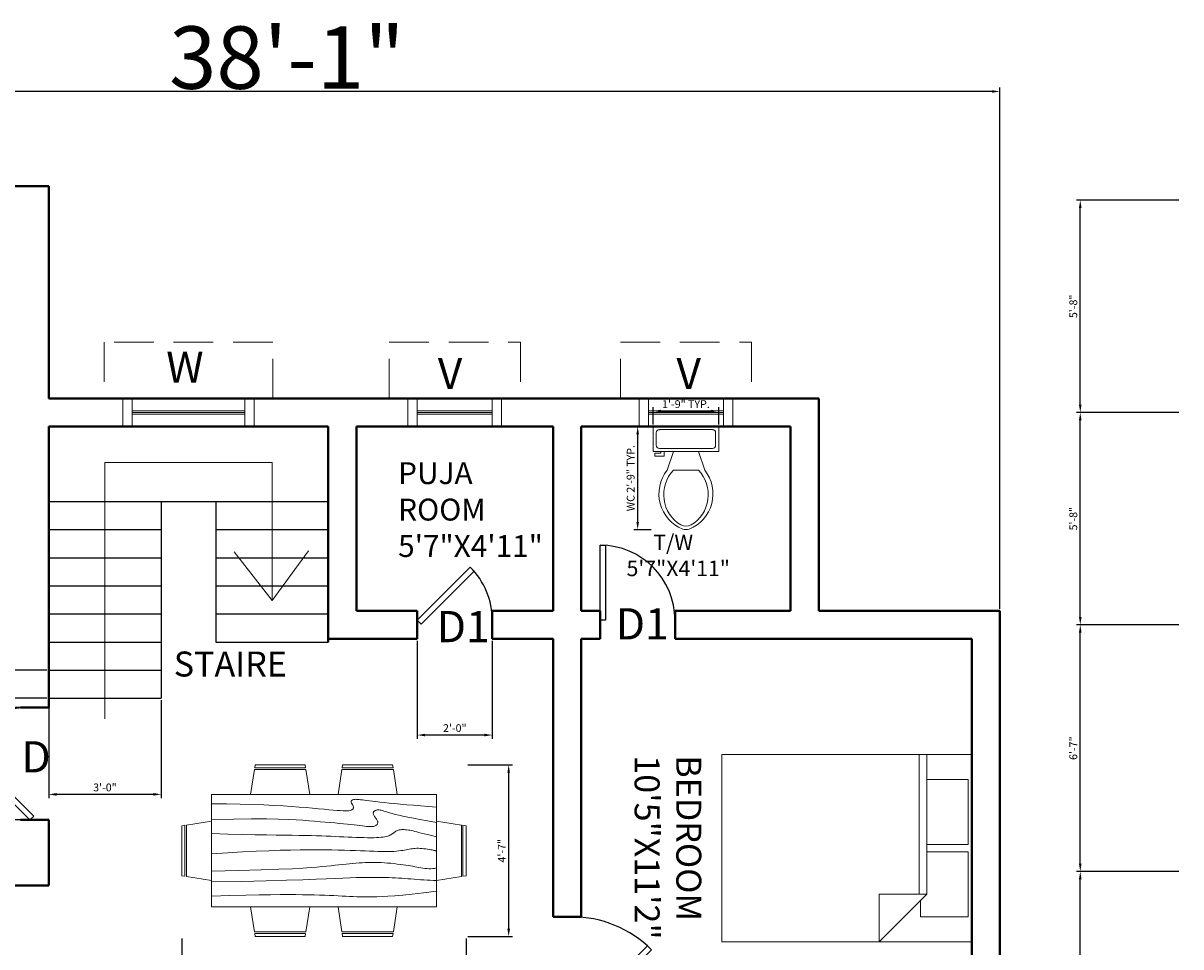
# Model space of a CAD drawing. Units: inches. Extents: x 4878 to 9282, y 5367 to 6617.
# Tile 6 of 14: x 5133 to 5503, y 6075 to 6371. Entities that reach past the tile are written whole.
import ezdxf

# ---------------------------------------------------------------- set-up
doc = ezdxf.new("R2010")
doc.units = ezdxf.units.IN
doc.linetypes.add('DASHED', pattern=[19.05, 12.7, -6.35])
for name, color, linetype, lineweight in [('A-ANNO-DIMS', 2, 'Continuous', 18), ('A-ANNO-SYMB', 2, 'Continuous', 18), ('A-ANNO-TEXT', 7, 'Continuous', 18), ('A-AREA-IDEN', 4, 'Continuous', 18), ('A-DOOR', 3, 'Continuous', 25), ('A-FLOR-FIXT', 9, 'Continuous', 20), ('A-FLOR-STRS', 7, 'Continuous', 25), ('A-FURN', 8, 'Continuous', 18), ('A-GLAZ', 30, 'Continuous', 20), ('A-ROOF-OVHD', 8, 'DASHED', 13), ('A-WALL', 7, 'Continuous', 40)]:
    doc.layers.add(name, color=color, linetype=linetype, lineweight=lineweight)
doc.styles.get("Standard").update_dxf_attribs({"font": 'arial.ttf'})
doc.dimstyles.new('ISO-25', dxfattribs={"dimtxt": 2.5, "dimasz": 2.5, "dimexe": 1.25, "dimexo": 0.625, "dimtad": 1, "dimdec": 0, "dimlunit": 3, "dimtxsty": 'Standard', "dimcen": 2.5, "dimadec": 0, "dimazin": 0, "dimtfac": 1, "dimtdec": 0, "dimtmove": 0, "dimatfit": 3, "dimfxl": 1, "dimarcsym": 0})

# ---------------------------------------------------------------- blocks, each defined once
blk = doc.blocks.new('Dining Set - 36 x 72 in.')
for p, q in [((-22.2343, 26.00059), (-23.4847, 17.99762)), ((-22.2304, 26), (-5.7608, 26)), ((-22, 27.5), (-22.1562, 26.50042)), ((-5.8416, 26.5), (-22.1534, 26.5)), ((-22, 27.5), (-6, 27.5)), ((-5.8437, 26.49966), (-6, 27.5)), ((-4.5152, 17.99762), (-5.7655, 25.99926)), ((5.7657, 26.00059), (4.5153, 17.99762)), ((5.7696, 26), (22.2392, 26)), ((6, 27.5), (5.8438, 26.50042)), ((22.1584, 26.5), (5.8466, 26.5)), ((6, 27.5), (22, 27.5)), ((22.1563, 26.49966), (22, 27.5)), ((23.4848, 17.99762), (22.2345, 25.99926)), ((36, 18), (-36, 18)), ((-36, 18), (-36, -18)), ((36, -18), (36, 18)), ((-45.5, 8), (-44.5004, 8.15617)), ((-45.5, 8), (-45.5, -8)), ((-44.5, -8.15843), (-44.5, 8.15338)), ((-44.0006, 8.23428), (-35.9976, 9.48474)), ((-44, 8.23041), (-44, -8.23915)), ((44.0006, 8.23428), (35.9976, 9.48474)), ((44, 8.23041), (44, -8.23915)), ((44.5, -8.15843), (44.5, 8.15338)), ((45.5, 8), (44.5005, 8.15617)), ((45.5, 8), (45.5, -8)), ((-44.4997, -8.15631), (-45.5, -8)), ((-35.9976, -9.48476), (-43.9993, -8.2345)), ((35.9976, -9.48476), (43.9993, -8.2345)), ((44.4997, -8.15631), (45.5, -8)), ((-36, -18), (36, -18)), ((-22.2343, -26.0006), (-23.4847, -17.99762)), ((-4.5152, -17.99762), (-5.7655, -25.99928)), ((5.7657, -26.0006), (4.5153, -17.99762)), ((23.4848, -17.99762), (22.2345, -25.99928)), ((-22.2304, -26), (-5.7608, -26)), ((-22, -27.5), (-22.1562, -26.50044)), ((-5.8416, -26.5), (-22.1534, -26.5)), ((-22, -27.5), (-6, -27.5)), ((-5.8437, -26.49967), (-6, -27.5)), ((5.7696, -26), (22.2392, -26)), ((6, -27.5), (5.8438, -26.50044)), ((22.1584, -26.5), (5.8466, -26.5)), ((6, -27.5), (22, -27.5)), ((22.1563, -26.49967), (22, -27.5))]:
    blk.add_line(p, q)
for points in [[(-36, 15), (-31.1772, 14.97754), (-26.8079, 14.91406), (-22.8538, 14.81543), (-19.276, 14.6875), (-16.0362, 14.53613), (-13.0957, 14.36718), (-10.4159, 14.18652), (-7.9583, 14), (-5.6904, 13.81315), (-3.6035, 13.63021), (-1.6954, 13.45508), (0.0365, 13.29166), (1.5945, 13.14388), (2.9811, 13.01562), (4.1988, 12.9108), (5.25, 12.83333), (6.1393, 12.78613), (6.8802, 12.76823), (7.4883, 12.77767), (7.9792, 12.8125), (8.3685, 12.87077), (8.6719, 12.95052), (8.9049, 13.0498), (9.0833, 13.16666), (9.2205, 13.29899), (9.3216, 13.44401), (9.3895, 13.59879), (9.4271, 13.76041), (9.4373, 13.92594), (9.4232, 14.09245), (9.3875, 14.257), (9.3333, 14.41666), (9.2638, 14.56917), (9.1836, 14.71484), (9.0975, 14.85465), (9.0104, 14.98958), (8.9272, 15.1206), (8.8529, 15.2487), (8.7922, 15.37483), (8.75, 15.5), (8.7305, 15.62467), (8.7344, 15.74739), (8.7617, 15.86621), (8.8125, 15.97916), (8.8867, 16.08431), (8.9844, 16.17968), (9.1055, 16.26334), (9.25, 16.33333), (9.4189, 16.38802), (9.6172, 16.42708), (9.8506, 16.45052), (10.125, 16.45833), (10.4463, 16.45052), (10.8203, 16.42708), (11.2529, 16.38802), (11.75, 16.33333), (12.3184, 16.26318), (12.9694, 16.17838), (13.7151, 16.07991), (14.5677, 15.96875), (15.5395, 15.84586), (16.6426, 15.71224), (17.8893, 15.56884), (19.2917, 15.41666), (20.859, 15.25667), (22.5879, 15.08984), (24.4721, 14.91715), (26.5052, 14.73958), (28.6809, 14.5581), (30.9929, 14.3737), (33.4347, 14.18733), (36, 14)], [(-36, 10), (-28.9766, 10.14274), (-23.1725, 10.20442), (-18.4241, 10.19775), (-14.5677, 10.13541), (-11.4399, 10.03011), (-8.877, 9.89453), (-6.7154, 9.74137), (-4.7917, 9.58333), (-2.9698, 9.43082), (-1.2246, 9.28515), (0.4415, 9.14534), (2.026, 9.01041), (3.5266, 8.87939), (4.9408, 8.7513), (6.266, 8.62516), (7.5, 8.5), (8.6411, 8.37549), (9.6914, 8.2539), (10.6538, 8.13818), (11.5312, 8.03125), (12.3267, 7.93603), (13.043, 7.85547), (13.6831, 7.79248), (14.25, 7.75), (14.7471, 7.7303), (15.1797, 7.73307), (15.5537, 7.75732), (15.875, 7.80208), (16.1494, 7.86637), (16.3828, 7.94922), (16.5811, 8.04964), (16.75, 8.16666), (16.8944, 8.29915), (17.0143, 8.44531), (17.1089, 8.60319), (17.1771, 8.77083), (17.218, 8.94629), (17.2305, 9.1276), (17.2137, 9.31282), (17.1667, 9.5), (17.0895, 9.6875), (16.987, 9.875), (16.8649, 10.0625), (16.7292, 10.25), (16.5856, 10.4375), (16.4401, 10.625), (16.2985, 10.8125), (16.1667, 11), (16.05, 11.18733), (15.9518, 11.3737), (15.8752, 11.5581), (15.8229, 11.73958), (15.798, 11.91715), (15.8034, 12.08984), (15.842, 12.25667), (15.9167, 12.41666), (16.0295, 12.56836), (16.1784, 12.70833), (16.3605, 12.83268), (16.5729, 12.9375), (16.8127, 13.01888), (17.0768, 13.07291), (17.3625, 13.0957), (17.6667, 13.08333), (17.9894, 13.03312), (18.3418, 12.94726), (18.7382, 12.82918), (19.1927, 12.68229), (19.7195, 12.51001), (20.3327, 12.31575), (21.0465, 12.10294), (21.875, 11.875), (22.8357, 11.63354), (23.959, 11.37304), (25.2786, 11.08618), (26.8282, 10.76562), (28.6414, 10.40405), (30.752, 9.99414), (33.1936, 9.52856), (36, 9)], [(-36, 5.5), (-30.7157, 5.3348), (-26.069, 5.20963), (-21.9946, 5.11767), (-18.4271, 5.05208), (-15.3009, 5.00602), (-12.5508, 4.97265), (-10.1112, 4.94515), (-7.9167, 4.91666), (-5.909, 4.88167), (-4.0586, 4.83984), (-2.3429, 4.79215), (-0.7396, 4.73958), (0.7739, 4.6831), (2.22, 4.6237), (3.6213, 4.56233), (5, 4.5), (6.373, 4.43782), (7.7344, 4.3776), (9.0723, 4.32129), (10.375, 4.27083), (11.6309, 4.22819), (12.8281, 4.19531), (13.9551, 4.17415), (15, 4.16666), (15.954, 4.17448), (16.819, 4.19791), (17.6001, 4.23698), (18.3021, 4.29166), (18.9299, 4.36198), (19.4883, 4.44791), (19.9823, 4.54948), (20.4167, 4.66666), (20.7969, 4.79899), (21.1302, 4.94401), (21.4245, 5.09879), (21.6875, 5.26041), (21.9271, 5.42594), (22.1511, 5.59245), (22.3672, 5.757), (22.5834, 5.91666), (22.8065, 6.06868), (23.0404, 6.21093), (23.2879, 6.34147), (23.5521, 6.45833), (23.8358, 6.55957), (24.142, 6.64323), (24.4735, 6.70735), (24.8334, 6.75), (25.2235, 6.76969), (25.642, 6.76692), (26.0858, 6.74267), (26.5521, 6.69791), (27.0379, 6.63362), (27.5404, 6.55078), (28.0565, 6.45036), (28.5834, 6.33333), (29.1242, 6.19987), (29.7071, 6.04687), (30.3661, 5.87044), (31.1354, 5.66666), (32.0493, 5.43164), (33.142, 5.16146), (34.4475, 4.85221), (36, 4.5)], [(-36, -1), (-30.7915, -0.6591), (-26.0195, -0.38216), (-21.6519, -0.16284), (-17.6563, 0.00521), (-14.0005, 0.12833), (-10.6523, 0.21289), (-7.5796, 0.26522), (-4.75, 0.29166), (-2.134, 0.29793), (0.2878, 0.28711), (2.5317, 0.26163), (4.6146, 0.22396), (6.5529, 0.17651), (8.3633, 0.12174), (10.0623, 0.06209), (11.6667, 0), (13.1899, -0.06201), (14.6341, -0.1211), (15.9982, -0.17432), (17.2813, -0.21875), (18.4823, -0.25147), (19.6003, -0.26953), (20.6343, -0.27002), (21.5834, -0.25), (22.4481, -0.20768), (23.2357, -0.14584), (23.9549, -0.06836), (24.6146, 0.02083), (25.2235, 0.11784), (25.7904, 0.21875), (26.3241, 0.31966), (26.8334, 0.41666), (27.3265, 0.50618), (27.8099, 0.58593), (28.2894, 0.65397), (28.7709, 0.70833), (29.2601, 0.74707), (29.763, 0.76823), (30.2855, 0.76985), (30.8334, 0.75), (31.4088, 0.70784), (31.9994, 0.64713), (32.589, 0.57275), (33.1615, 0.48958), (33.7008, 0.4025), (34.1908, 0.3164), (34.6153, 0.23616), (34.9584, 0.16666), (35.2099, 0.11165), (35.3848, 0.07031), (35.504, 0.04069), (35.5886, 0.02083), (35.6594, 0.00879), (35.7377, 0.0026), (35.8442, 0.00032), (36, 0)], [(-36, -6.5), (-27.1843, -6.31267), (-20.084, -6.1263), (-14.469, -5.9419), (-10.1094, -5.76042), (-6.7752, -5.58285), (-4.2363, -5.41016), (-2.2629, -5.24333), (-0.625, -5.08334), (0.8708, -4.93099), (2.2715, -4.78646), (3.5872, -4.64974), (4.8281, -4.52084), (6.0046, -4.39974), (7.127, -4.28646), (8.2053, -4.18099), (9.25, -4.08334), (10.2705, -3.99382), (11.2734, -3.91407), (12.2647, -3.84603), (13.25, -3.79167), (14.2354, -3.75293), (15.2266, -3.73177), (16.2295, -3.73015), (17.25, -3.75), (18.2912, -3.79248), (19.3451, -3.85547), (20.4009, -3.93604), (21.4479, -4.03125), (22.4754, -4.13819), (23.4727, -4.25391), (24.4289, -4.37549), (25.3334, -4.5), (26.1785, -4.62492), (26.9694, -4.74935), (27.7145, -4.87281), (28.4219, -4.99479), (29.1, -5.11483), (29.7572, -5.23242), (30.4016, -5.34709), (31.0417, -5.45834), (31.6837, -5.56437), (32.3262, -5.65821), (32.9658, -5.73153), (33.599, -5.77604), (34.2224, -5.78345), (34.8327, -5.74545), (35.4264, -5.65373), (36, -5.5)], [(-36, -10), (-26.4022, -9.81299), (-18.4675, -9.62891), (-11.9839, -9.45069), (-6.7396, -9.28125), (-2.5226, -9.12354), (0.8789, -8.98047), (3.6769, -8.85498), (6.0833, -8.75), (8.2767, -8.66765), (10.3021, -8.60677), (12.1712, -8.56543), (13.8958, -8.54167), (15.4876, -8.53353), (16.9583, -8.53907), (18.3197, -8.55632), (19.5834, -8.58334), (20.7616, -8.61841), (21.8685, -8.66081), (22.9188, -8.71004), (23.9271, -8.76563), (24.9081, -8.82707), (25.8763, -8.89388), (26.8465, -8.96558), (27.8334, -9.04167), (28.8474, -9.12118), (29.8828, -9.20117), (30.93, -9.27824), (31.9792, -9.34896), (33.0205, -9.40991), (34.0443, -9.45768), (35.0407, -9.48885), (36, -9.5)], [(-36, -14.5), (-30.0881, -14.33513), (-25.0332, -14.21224), (-20.7312, -14.12647), (-17.0781, -14.07292), (-13.97, -14.04671), (-11.3027, -14.04297), (-8.9724, -14.05681), (-6.875, -14.08334), (-4.9224, -14.11833), (-3.0905, -14.16016), (-1.3709, -14.20785), (0.2448, -14.26042), (1.7647, -14.3169), (3.1973, -14.3763), (4.5507, -14.43767), (5.8333, -14.5), (7.0554, -14.5621), (8.235, -14.62175), (9.3922, -14.67652), (10.5469, -14.72396), (11.7192, -14.76164), (12.929, -14.78711), (14.1965, -14.79794), (15.5417, -14.79167), (16.9933, -14.76424), (18.6152, -14.70508), (20.4804, -14.60197), (22.6615, -14.44271), (25.2312, -14.21509), (28.2624, -13.9069), (31.8277, -13.50594), (36, -13)]]:
    blk.add_lwpolyline(points)
blk = doc.blocks.new('Bed - Queen')
for p, q in [((0, -80.00003), (0, 0)), ((0, 0), (59.99999, 0)), ((59.99999, 0), (59.99999, -80.00003)), ((7.99999, -1.2), (28.79998, -1.2)), ((7.99999, -14.4), (7.99999, -1.2)), ((28.79998, -1.2), (28.79998, -14.4)), ((31.19999, -1.2), (51.99999, -1.2)), ((31.19999, -14.4), (31.19999, -1.2)), ((51.99999, -1.2), (51.99999, -16.4)), ((0, -14.4), (44.8, -14.4)), ((59.99999, -29.6), (44.8, -14.4)), ((44.8, -14.4), (44.8, -29.6)), ((44.8, -16.8), (0, -16.8)), ((51.99999, -16.4), (46.79936, -16.4)), ((44.8, -29.6), (59.99999, -29.6)), ((59.99999, -80.00003), (0, -80.00003))]:
    blk.add_line(p, q)
blk = doc.blocks.new('Toilet - top')
for p, q in [((9.5, -6), (9.5, -2)), ((-10, -8.5), (-8, -8.5)), ((-10, -9.5), (-10, -8.5)), ((-7, -9.5), (-10, -9.5)), ((-8, -8.5), (-8, -8)), ((-7, -8), (-7, -9.5)), ((-4, -8), (-6, -14)), ((4, -8), (6, -14)), ((4, -14), (-4, -14))]:
    blk.add_line(p, q)
blk.add_lwpolyline([(10.5, -8), (10.5, 0), (-10.5, 0), (-10.5, -8)], close=True)
for points in [[(-9.5, -2), (-9.5, -6)], [(8.5, -1), (-8.5, -1)], [(-8.5, -7), (8.5, -7)]]:
    blk.add_lwpolyline(points)
for centre, radius, start, end in [((-8.62, -1.88), 0.884, 81.8699, 188.1301), ((8.62, -1.88), 0.884, 351.8699, 98.1301), ((-8.62, -6.12), 0.884, 171.8699, 278.1301), ((8.62, -6.12), 0.884, 261.8699, 8.1301), ((3.52, -21.58), 12.17, 141.4691, 247.9714), ((4.2, -21.82), 11.33, 136.3677, 238.9468), ((-3.52, -21.58), 12.17, 292.0284, 38.5307), ((-4.2, -21.82), 11.33, 301.053, 43.6321), ((0, -27.88), 4, 245.7318, 294.2682), ((0, -29), 4, 254.8605, 285.1395)]:
    blk.add_arc(centre, radius, start, end)
blk = doc.blocks.new('*U10')
for p, q in [((0, 0), (0, -6)), ((24, 0), (24, -6))]:
    blk.add_line(p, q)
blk.add_lwpolyline([(0, 0), (16.97, 16.97), (18.21, 15.73), (1.24, -1.24)], close=True)
blk.add_arc((0, 0), 24, 0, 45)
blk = doc.blocks.new('*U15')
for p, q in [((0, 0), (0, -6)), ((24, 0), (24, -6))]:
    blk.add_line(p, q)
blk.add_lwpolyline([(0, 0), (0, 24), (1.75, 24), (1.75, 0)], close=True)
blk.add_arc((0, 0), 24, 0, 90)
blk = doc.blocks.new('*U8')
for p, q in [((-36, 0), (-36, 6)), ((0, 0), (0, 6))]:
    blk.add_line(p, q)
blk.add_lwpolyline([(0, 0), (-25.46, -25.46), (-26.69, -24.22), (-1.24, 1.24)], close=True)
blk.add_arc((0, 0), 36, 180, 225)
blk = doc.blocks.new('*U13')
for p, q in [((0, 0), (0, -6)), ((-36, 0), (-36, -6))]:
    blk.add_line(p, q)
blk.add_lwpolyline([(0, 0), (-25.46, 25.46), (-26.69, 24.22), (-1.24, -1.24)], close=True)
blk.add_arc((0, 0), 36, 135, 180)
blk = doc.blocks.new('*D16')
at = {"layer": 'A-ANNO-DIMS', "color": 0, "lineweight": -2, "transparency": 16777216}
for p, q in [((4988.98, 6183.27), (4988.98, 6350.19)), ((5442.98, 6348.94), (4991.48, 6348.94)), ((5445.48, 6183.27), (5445.48, 6350.19))]:
    blk.add_line(p, q, dxfattribs=at)
at = {"layer": 'A-ANNO-DIMS', "color": 0, "transparency": 16777216}
for points in [[(4991.48, 6349.36), (4991.48, 6348.53), (4988.98, 6348.94)], [(5442.98, 6349.36), (5442.98, 6348.53), (5445.48, 6348.94)]]:
    blk.add_solid(points, dxfattribs=at)
at = {"layer": 'Defpoints', "color": 0, "transparency": 16777216}
for p in [(4988.98, 6348.94), (4988.98, 6182.64), (5445.48, 6182.64)]:
    blk.add_point(p, dxfattribs=at)
at = {"layer": 'A-ANNO-DIMS', "color": 0, "transparency": 16777216, "insert": (5217.23, 6359.79), "char_height": 2.5, "attachment_point": 5}
blk.add_mtext('{\\H8x;38\'-1"}', dxfattribs=at)
blk = doc.blocks.new('WINDOW-PLAN-36IN')
for p, q in [((0, 0), (0, 9)), ((3, 0), (3, 9)), ((39, 0), (39, 9)), ((42, 0), (42, 9)), ((3, 5), (39, 5)), ((3, 4.5), (39, 4.5)), ((3, 4), (39, 4))]:
    blk.add_line(p, q)
blk = doc.blocks.new('WINDOW-PLAN-24IN')
for p, q in [((9, 30), (0, 30)), ((9, 27), (0, 27)), ((4, 3), (4, 27)), ((4.5, 3), (4.5, 27)), ((5, 3), (5, 27)), ((9, 3), (0, 3)), ((9, 0), (0, 0))]:
    blk.add_line(p, q)
blk = doc.blocks.new('WINDOW-HOOD-54IN')
for p, q in [((0, 18), (0, 0)), ((54, 0), (54, 18)), ((0, 0), (54, 0))]:
    blk.add_line(p, q)
blk = doc.blocks.new('WINDOW-HOOD-42IN')
for p, q in [((18, 42), (0, 42)), ((0, 42), (0, 0)), ((0, 0), (18, 0))]:
    blk.add_line(p, q)
blk = doc.blocks.new('*D55')
at = {"layer": 'A-ANNO-DIMS', "color": 0, "lineweight": -2, "transparency": 16777216}
for p, q in [((5333.85, 6241.64), (5328.27, 6241.64)), ((5329.52, 6211.1), (5329.52, 6239.14)), ((5333.85, 6208.6), (5328.27, 6208.6))]:
    blk.add_line(p, q, dxfattribs=at)
at = {"layer": 'A-ANNO-DIMS', "color": 0, "transparency": 16777216}
for points in [[(5329.1, 6239.14), (5329.94, 6239.14), (5329.52, 6241.64)], [(5329.1, 6211.1), (5329.94, 6211.1), (5329.52, 6208.6)]]:
    blk.add_solid(points, dxfattribs=at)
at = {"layer": 'Defpoints', "color": 0, "transparency": 16777216}
for p in [(5329.52, 6241.64), (5334.48, 6241.64), (5334.48, 6208.6)]:
    blk.add_point(p, dxfattribs=at)
at = {"layer": 'A-ANNO-DIMS', "color": 0, "transparency": 16777216, "insert": (5327.6, 6225.12), "char_height": 2.5, "attachment_point": 5, "rotation": 90}
blk.add_mtext('WC 2\'-9" TYP.', dxfattribs=at)
blk = doc.blocks.new('*D56')
at = {"layer": 'A-ANNO-DIMS', "color": 0, "lineweight": -2, "transparency": 16777216}
for p, q in [((5334.48, 6242.27), (5334.48, 6247.85)), ((5336.98, 6246.6), (5352.98, 6246.6)), ((5355.48, 6242.27), (5355.48, 6247.85))]:
    blk.add_line(p, q, dxfattribs=at)
at = {"layer": 'A-ANNO-DIMS', "color": 0, "transparency": 16777216}
for points in [[(5336.98, 6247.02), (5336.98, 6246.19), (5334.48, 6246.6)], [(5352.98, 6247.02), (5352.98, 6246.19), (5355.48, 6246.6)]]:
    blk.add_solid(points, dxfattribs=at)
at = {"layer": 'Defpoints', "color": 0, "transparency": 16777216}
for p in [(5355.48, 6246.6), (5334.48, 6241.64), (5355.48, 6241.64)]:
    blk.add_point(p, dxfattribs=at)
at = {"layer": 'A-ANNO-DIMS', "color": 0, "transparency": 16777216, "insert": (5344.98, 6248.5), "char_height": 2.5, "attachment_point": 5}
blk.add_mtext('1\'-9" TYP.', dxfattribs=at)
blk = doc.blocks.new('*D61')
at = {"layer": 'A-ANNO-DIMS', "color": 0, "lineweight": -2, "transparency": 16777216}
for p, q in [((5183.58, 6077.68), (5183.58, 6063.4)), ((5274.58, 6077.68), (5274.58, 6063.4)), ((5186.08, 6064.65), (5272.08, 6064.65))]:
    blk.add_line(p, q, dxfattribs=at)
at = {"layer": 'A-ANNO-DIMS', "color": 0, "transparency": 16777216}
for points in [[(5186.08, 6065.07), (5186.08, 6064.23), (5183.58, 6064.65)], [(5272.08, 6065.07), (5272.08, 6064.23), (5274.58, 6064.65)]]:
    blk.add_solid(points, dxfattribs=at)
at = {"layer": 'Defpoints', "color": 0, "transparency": 16777216}
for p in [(5183.58, 6078.3), (5274.58, 6078.3), (5274.58, 6064.65)]:
    blk.add_point(p, dxfattribs=at)
at = {"layer": 'A-ANNO-DIMS', "color": 0, "transparency": 16777216, "insert": (5229.08, 6066.57), "char_height": 2.5, "attachment_point": 5}
blk.add_mtext('DINING SET 7\'-7"', dxfattribs=at)
blk = doc.blocks.new('*D62')
at = {"layer": 'A-ANNO-DIMS', "color": 0, "lineweight": -2, "transparency": 16777216}
for p, q in [((5275.2, 6133.3), (5289.48, 6133.3)), ((5288.23, 6080.8), (5288.23, 6130.8)), ((5275.2, 6078.3), (5289.48, 6078.3))]:
    blk.add_line(p, q, dxfattribs=at)
at = {"layer": 'A-ANNO-DIMS', "color": 0, "transparency": 16777216}
for points in [[(5287.81, 6130.8), (5288.64, 6130.8), (5288.23, 6133.3)], [(5287.81, 6080.8), (5288.64, 6080.8), (5288.23, 6078.3)]]:
    blk.add_solid(points, dxfattribs=at)
at = {"layer": 'Defpoints', "color": 0, "transparency": 16777216}
for p in [(5274.58, 6133.3), (5288.23, 6133.3), (5274.58, 6078.3)]:
    blk.add_point(p, dxfattribs=at)
at = {"layer": 'A-ANNO-DIMS', "color": 0, "transparency": 16777216, "insert": (5286.35, 6105.8), "char_height": 2.5, "attachment_point": 5, "rotation": 90}
blk.add_mtext('4\'-7"', dxfattribs=at)
blk = doc.blocks.new('*D74')
at = {"layer": 'A-ANNO-DIMS', "color": 0, "lineweight": -2, "transparency": 16777216}
for p, q in [((5502.78, 6099.14), (5469.95, 6099.14)), ((5471.2, 6037.64), (5471.2, 6096.64)), ((5502.78, 6035.14), (5469.95, 6035.14))]:
    blk.add_line(p, q, dxfattribs=at)
at = {"layer": 'A-ANNO-DIMS', "color": 0, "transparency": 16777216}
for points in [[(5470.79, 6096.64), (5471.62, 6096.64), (5471.2, 6099.14)], [(5470.79, 6037.64), (5471.62, 6037.64), (5471.2, 6035.14)]]:
    blk.add_solid(points, dxfattribs=at)
at = {"layer": 'Defpoints', "color": 0, "transparency": 16777216}
for p in [(5471.2, 6099.14), (5503.4, 6099.14), (5503.4, 6035.14)]:
    blk.add_point(p, dxfattribs=at)
at = {"layer": 'A-ANNO-DIMS', "color": 0, "transparency": 16777216, "insert": (5469.31, 6067.14), "char_height": 2.5, "attachment_point": 5, "rotation": 90}
blk.add_mtext('5\'-4"', dxfattribs=at)
blk = doc.blocks.new('*D75')
at = {"layer": 'A-ANNO-DIMS', "color": 0, "lineweight": -2, "transparency": 16777216}
for p, q in [((5502.78, 6178.14), (5469.95, 6178.14)), ((5471.2, 6101.64), (5471.2, 6175.64)), ((5502.78, 6099.14), (5469.95, 6099.14))]:
    blk.add_line(p, q, dxfattribs=at)
at = {"layer": 'A-ANNO-DIMS', "color": 0, "transparency": 16777216}
for points in [[(5470.79, 6175.64), (5471.62, 6175.64), (5471.2, 6178.14)], [(5470.79, 6101.64), (5471.62, 6101.64), (5471.2, 6099.14)]]:
    blk.add_solid(points, dxfattribs=at)
at = {"layer": 'Defpoints', "color": 0, "transparency": 16777216}
for p in [(5471.2, 6178.14), (5503.4, 6178.14), (5503.4, 6099.14)]:
    blk.add_point(p, dxfattribs=at)
at = {"layer": 'A-ANNO-DIMS', "color": 0, "transparency": 16777216, "insert": (5469.3, 6138.64), "char_height": 2.5, "attachment_point": 5, "rotation": 90}
blk.add_mtext('6\'-7"', dxfattribs=at)
blk = doc.blocks.new('*D76')
at = {"layer": 'A-ANNO-DIMS', "color": 0, "lineweight": -2, "transparency": 16777216}
for p, q in [((5502.78, 6246.14), (5469.95, 6246.14)), ((5471.2, 6180.64), (5471.2, 6243.64)), ((5502.78, 6178.14), (5469.95, 6178.14))]:
    blk.add_line(p, q, dxfattribs=at)
at = {"layer": 'A-ANNO-DIMS', "color": 0, "transparency": 16777216}
for points in [[(5470.79, 6243.64), (5471.62, 6243.64), (5471.2, 6246.14)], [(5470.79, 6180.64), (5471.62, 6180.64), (5471.2, 6178.14)]]:
    blk.add_solid(points, dxfattribs=at)
at = {"layer": 'Defpoints', "color": 0, "transparency": 16777216}
for p in [(5471.2, 6246.14), (5503.4, 6246.14), (5503.4, 6178.14)]:
    blk.add_point(p, dxfattribs=at)
at = {"layer": 'A-ANNO-DIMS', "color": 0, "transparency": 16777216, "insert": (5469.3, 6212.14), "char_height": 2.5, "attachment_point": 5, "rotation": 90}
blk.add_mtext('5\'-8"', dxfattribs=at)
blk = doc.blocks.new('*D77')
at = {"layer": 'A-ANNO-DIMS', "color": 0, "lineweight": -2, "transparency": 16777216}
for p, q in [((5502.78, 6314.14), (5469.95, 6314.14)), ((5471.2, 6248.64), (5471.2, 6311.64)), ((5502.78, 6246.14), (5469.95, 6246.14))]:
    blk.add_line(p, q, dxfattribs=at)
at = {"layer": 'A-ANNO-DIMS', "color": 0, "transparency": 16777216}
for points in [[(5470.79, 6311.64), (5471.62, 6311.64), (5471.2, 6314.14)], [(5470.79, 6248.64), (5471.62, 6248.64), (5471.2, 6246.14)]]:
    blk.add_solid(points, dxfattribs=at)
at = {"layer": 'Defpoints', "color": 0, "transparency": 16777216}
for p in [(5471.2, 6314.14), (5503.4, 6314.14), (5503.4, 6246.14)]:
    blk.add_point(p, dxfattribs=at)
at = {"layer": 'A-ANNO-DIMS', "color": 0, "transparency": 16777216, "insert": (5469.3, 6280.14), "char_height": 2.5, "attachment_point": 5, "rotation": 90}
blk.add_mtext('5\'-8"', dxfattribs=at)
blk = doc.blocks.new('*D105')
at = {"layer": 'A-ANNO-DIMS', "color": 0, "lineweight": -2, "transparency": 16777216}
for p, q in [((5140.35, 6151.64), (5108.93, 6151.64)), ((5110.18, 6118.14), (5110.18, 6149.14)), ((5140.35, 6115.64), (5108.93, 6115.64))]:
    blk.add_line(p, q, dxfattribs=at)
at = {"layer": 'A-ANNO-DIMS', "color": 0, "transparency": 16777216}
for points in [[(5109.76, 6149.14), (5110.59, 6149.14), (5110.18, 6151.64)], [(5109.76, 6118.14), (5110.59, 6118.14), (5110.18, 6115.64)]]:
    blk.add_solid(points, dxfattribs=at)
at = {"layer": 'Defpoints', "color": 0, "transparency": 16777216}
for p in [(5110.18, 6151.64), (5140.98, 6151.64), (5140.98, 6115.64)]:
    blk.add_point(p, dxfattribs=at)
at = {"layer": 'A-ANNO-DIMS', "color": 0, "transparency": 16777216, "insert": (5108.27, 6133.64), "char_height": 2.5, "attachment_point": 5, "rotation": 90}
blk.add_mtext('3\'-0"', dxfattribs=at)
blk = doc.blocks.new('*D106')
at = {"layer": 'A-ANNO-DIMS', "color": 0, "lineweight": -2, "transparency": 16777216}
for p, q in [((5258.98, 6173.02), (5258.98, 6141.59)), ((5282.98, 6173.02), (5282.98, 6141.59)), ((5280.48, 6142.84), (5261.48, 6142.84))]:
    blk.add_line(p, q, dxfattribs=at)
at = {"layer": 'A-ANNO-DIMS', "color": 0, "transparency": 16777216}
for points in [[(5261.48, 6143.26), (5261.48, 6142.43), (5258.98, 6142.84)], [(5280.48, 6143.26), (5280.48, 6142.43), (5282.98, 6142.84)]]:
    blk.add_solid(points, dxfattribs=at)
at = {"layer": 'Defpoints', "color": 0, "transparency": 16777216}
for p in [(5258.98, 6173.64), (5282.98, 6173.64), (5258.98, 6142.84)]:
    blk.add_point(p, dxfattribs=at)
at = {"layer": 'A-ANNO-DIMS', "color": 0, "transparency": 16777216, "insert": (5270.98, 6144.75), "char_height": 2.5, "attachment_point": 5}
blk.add_mtext('2\'-0"', dxfattribs=at)
blk = doc.blocks.new('*D113')
at = {"layer": 'A-ANNO-DIMS', "color": 0, "lineweight": -2, "transparency": 16777216}
for p, q in [((5140.98, 6154.02), (5140.98, 6122.59)), ((5176.98, 6154.02), (5176.98, 6122.59)), ((5174.48, 6123.84), (5143.48, 6123.84))]:
    blk.add_line(p, q, dxfattribs=at)
at = {"layer": 'A-ANNO-DIMS', "color": 0, "transparency": 16777216}
for points in [[(5143.48, 6124.26), (5143.48, 6123.43), (5140.98, 6123.84)], [(5174.48, 6124.26), (5174.48, 6123.43), (5176.98, 6123.84)]]:
    blk.add_solid(points, dxfattribs=at)
at = {"layer": 'Defpoints', "color": 0, "transparency": 16777216}
for p in [(5140.98, 6154.64), (5176.98, 6154.64), (5140.98, 6123.84)]:
    blk.add_point(p, dxfattribs=at)
at = {"layer": 'A-ANNO-DIMS', "color": 0, "transparency": 16777216, "insert": (5158.98, 6125.75), "char_height": 2.5, "attachment_point": 5}
blk.add_mtext('3\'-0"', dxfattribs=at)
blk = doc.blocks.new('*D114')
at = {"layer": 'A-ANNO-DIMS', "color": 0, "lineweight": -2, "transparency": 16777216}
for p, q in [((5140.35, 6163.64), (4938.93, 6163.64)), ((4940.18, 6161.14), (4940.18, 6157.14)), ((5140.35, 6154.64), (4938.93, 6154.64))]:
    blk.add_line(p, q, dxfattribs=at)
at = {"layer": 'A-ANNO-DIMS', "color": 0, "transparency": 16777216}
for points in [[(4939.76, 6161.14), (4940.59, 6161.14), (4940.18, 6163.64)], [(4939.76, 6157.14), (4940.59, 6157.14), (4940.18, 6154.64)]]:
    blk.add_solid(points, dxfattribs=at)
at = {"layer": 'Defpoints', "color": 0, "transparency": 16777216}
for p in [(5140.98, 6163.64), (4940.18, 6154.64), (5140.98, 6154.64)]:
    blk.add_point(p, dxfattribs=at)
at = {"layer": 'A-ANNO-DIMS', "color": 0, "transparency": 16777216, "insert": (4938.28, 6159.14), "char_height": 2.5, "attachment_point": 5, "rotation": 90}
blk.add_mtext('0\'-9"', dxfattribs=at)

msp = doc.modelspace()

# ---------------------------------------------------------------- linework, layer by layer
at = {"layer": 'A-ANNO-SYMB'}
for p, q in [((5158.98, 6148.02), (5158.98, 6230.17)), ((5158.98, 6230.17), (5212.48, 6230.17)), ((5212.48, 6230.17), (5212.48, 6185.94)), ((5212.48, 6185.94), (5200.37, 6201.49)), ((5212.48, 6185.94), (5224.12, 6201.83))]:
    msp.add_line(p, q, dxfattribs=at)
at = {"layer": 'A-FLOR-STRS'}
for p, q in [((5140.98, 6217.64), (5230.48, 6217.64)), ((5176.98, 6217.64), (5176.98, 6154.64)), ((5194.48, 6217.64), (5194.48, 6172.64)), ((5140.98, 6208.64), (5176.98, 6208.64)), ((5194.48, 6208.64), (5230.48, 6208.64)), ((5140.98, 6199.64), (5176.98, 6199.64)), ((5194.48, 6199.64), (5230.48, 6199.64)), ((5140.98, 6190.64), (5176.98, 6190.64)), ((5194.48, 6190.64), (5230.48, 6190.64)), ((5140.98, 6181.64), (5176.98, 6181.64)), ((5194.48, 6181.64), (5230.48, 6181.64)), ((5140.98, 6172.64), (5176.98, 6172.64)), ((5194.48, 6172.64), (5230.48, 6172.64)), ((5140.98, 6163.64), (5176.98, 6163.64)), ((5140.98, 6154.64), (5176.98, 6154.64))]:
    msp.add_line(p, q, dxfattribs=at)
at = {"layer": 'A-WALL'}
for p, q in [((5043.98, 6318.64), (5140.98, 6318.64)), ((5140.98, 6318.64), (5140.98, 6250.64)), ((5140.98, 6250.64), (5387.48, 6250.64)), ((5387.48, 6250.64), (5387.48, 6182.64)), ((5140.98, 6241.64), (5230.48, 6241.64)), ((5140.98, 6241.64), (5140.98, 6151.64)), ((5230.48, 6241.64), (5230.48, 6172.64)), ((5239.48, 6241.64), (5239.48, 6182.64)), ((5239.48, 6241.64), (5302.48, 6241.64)), ((5302.48, 6241.64), (5302.48, 6182.64)), ((5311.48, 6241.64), (5311.48, 6182.64)), ((5311.48, 6241.64), (5378.48, 6241.64)), ((5378.48, 6241.64), (5378.48, 6182.64)), ((5239.48, 6182.64), (5258.98, 6182.64)), ((5258.98, 6182.64), (5258.98, 6173.64)), ((5282.98, 6182.64), (5282.98, 6173.64)), ((5282.98, 6182.64), (5302.48, 6182.64)), ((5311.48, 6182.64), (5317.48, 6182.64)), ((5317.48, 6182.64), (5317.48, 6173.64)), ((5341.48, 6182.64), (5341.48, 6173.64)), ((5341.48, 6182.64), (5378.48, 6182.64)), ((5387.48, 6182.64), (5445.48, 6182.64)), ((5445.48, 6182.64), (5445.48, 6030.64)), ((5230.48, 6173.64), (5258.98, 6173.64)), ((5282.98, 6173.64), (5302.48, 6173.64)), ((5302.48, 6173.64), (5302.48, 6084.64)), ((5311.48, 6173.64), (5311.48, 6084.64)), ((5311.48, 6173.64), (5317.48, 6173.64)), ((5341.48, 6173.64), (5436.48, 6173.64)), ((5436.48, 6173.64), (5436.48, 6039.64)), ((5131.98, 6151.64), (5140.98, 6151.64)), ((5131.98, 6115.64), (5140.98, 6115.64)), ((5140.98, 6115.64), (5140.98, 6094.64)), ((5140.98, 6094.64), (5085.98, 6094.64)), ((5311.48, 6084.64), (5302.48, 6084.64))]:
    msp.add_line(p, q, dxfattribs=at)

# ---------------------------------------------------------------- block references
at = {"layer": 'A-DOOR'}
for name, p in [('*U15', (5317.48, 6179.64)), ('*U10', (5258.98, 6179.64))]:
    msp.add_blockref(name, p, dxfattribs=at)
at = {"layer": 'A-DOOR', "rotation": 270}
for name, p in [('*U8', (5134.98, 6115.64)), ('*U13', (5308.48, 6048.64))]:
    msp.add_blockref(name, p, dxfattribs=at)
at = {"layer": 'A-FLOR-FIXT'}
msp.add_blockref('Toilet - top', (5344.98, 6241.64), dxfattribs=at)
at = {"layer": 'A-FURN', "rotation": 270}
msp.add_blockref('Bed - Queen', (5436.48, 6136.64), dxfattribs=at)
at = {"layer": 'A-FURN'}
msp.add_blockref('Dining Set - 36 x 72 in.', (5229.08, 6105.8), dxfattribs=at)
at = {"layer": 'A-GLAZ'}
msp.add_blockref('WINDOW-PLAN-36IN', (5164.73, 6241.65), dxfattribs=at)
at = {"layer": 'A-GLAZ', "extrusion": (0, 0, -1), "zscale": -1, "rotation": 90}
for p in [(-5255.98, 6241.64), (-5329.98, 6241.64)]:
    msp.add_blockref('WINDOW-PLAN-24IN', p, dxfattribs=at)
at = {"layer": 'A-ROOF-OVHD', "rotation": 180}
msp.add_blockref('WINDOW-HOOD-54IN', (5212.73, 6268.64), dxfattribs=at)
at = {"layer": 'A-ROOF-OVHD', "extrusion": (0, 0, -1), "zscale": -1, "rotation": 270}
for p in [(-5291.98, 6268.64), (-5365.98, 6268.64)]:
    msp.add_blockref('WINDOW-HOOD-42IN', p, dxfattribs=at)

# ---------------------------------------------------------------- texts
at = {"layer": 'A-ANNO-TEXT', "char_height": 10, "width": 649.8744, "attachment_point": 1}
for s, insert in [('W', (5178.59, 6265.67)), ('V', (5265.53, 6263.64)), ('V', (5341.92, 6263.61)), ('D1', (5265.19, 6182.58)), ('D1', (5322.5, 6183.46)), ('D', (5132.25, 6140.88))]:
    msp.add_mtext(s, dxfattribs=dict(at, insert=insert))
at = {"layer": 'A-ANNO-TEXT', "insert": (5181.01, 6169.59), "char_height": 8, "attachment_point": 1}
msp.add_mtext_dynamic_manual_height_columns('STAIRE', width=123.3151, gutter_width=12.5, heights=[0], dxfattribs=at)
at = {"layer": 'A-AREA-IDEN', "char_height": 7, "attachment_point": 1}
for s, width, insert in [('PUJA \\PROOM\\P5\'7"X4\'11"', 312.5956, (5252.84, 6230.21)), ('    {\\H0.71429x;T/W\\P5\'7"X4\'11"}', 337.032, (5325.96, 6207.06))]:
    msp.add_mtext_dynamic_manual_height_columns(s, width=width, gutter_width=12.5, heights=[0], dxfattribs=dict(at, insert=insert))
at = {"layer": 'A-AREA-IDEN', "insert": (5349.88, 6136.35), "char_height": 8, "attachment_point": 1, "rotation": 270}
msp.add_mtext_dynamic_manual_height_columns('BEDROOM\\P10\'5"X11\'2"', width=364.6117, gutter_width=12.5, heights=[0], dxfattribs=at)

# ---------------------------------------------------------------- dimensions: what is measured, and where the dimension line sits
at = {"layer": 'A-ANNO-DIMS'}
for base, p1, p2, text, override, picture, middle in [((4988.97709281, 6348.94354297), (5445.47709281, 6182.64478635), (4988.97709281, 6182.64478635), '{\\H8x;<>}', {"dimclrd": 0, "dimclre": 0, "dimclrt": 0}, '*D16', (5217.22709281, 6359.786824)), ((5355.48, 6246.6), (5334.48, 6241.64), (5355.48, 6241.64), '<> TYP.', {"dimdec": 1, "dimlfac": 1, "dimrnd": 0, "dimzin": 1, "dimdsep": 46, "dimlunit": 4, "dimfrac": 2}, '*D56', (5344.98, 6248.5)), ((5274.58, 6064.65), (5183.58, 6078.3), (5274.58, 6078.3), 'DINING SET <>', {"dimdec": 1, "dimlfac": 1, "dimrnd": 0, "dimzin": 1, "dimdsep": 46, "dimlunit": 4, "dimfrac": 2}, '*D61', (5229.08, 6066.57))]:
    dim = msp.add_linear_dim(base=base, p1=p1, p2=p2, text=text, dimstyle='ISO-25', override=override, dxfattribs=at)
    dim.commit()
    dim.dimension.update_dxf_attribs({"geometry": picture, "text_midpoint": middle})
for base, p1, p2, angle, picture, middle in [((5471.2, 6314.14), (5503.4, 6246.14), (5503.4, 6314.14), 90, '*D77', (5469.3, 6280.14)), ((5471.2, 6246.14), (5503.4, 6178.14), (5503.4, 6246.14), 90, '*D76', (5469.3, 6212.14)), ((5471.2, 6178.14), (5503.4, 6099.14), (5503.4, 6178.14), 90, '*D75', (5469.3, 6138.64)), ((5258.98, 6142.84), (5282.98, 6173.64), (5258.98, 6173.64), 180, '*D106', (5270.98, 6144.75)), ((4940.18, 6154.64), (5140.98, 6163.64), (5140.98, 6154.64), 90, '*D114', (4938.28, 6159.14)), ((5140.98, 6123.84), (5176.98, 6154.64), (5140.98, 6154.64), 180, '*D113', (5158.98, 6125.75)), ((5110.18, 6151.64), (5140.98, 6115.64), (5140.98, 6151.64), 90, '*D105', (5108.27, 6133.64)), ((5288.23, 6133.3), (5274.58, 6078.3), (5274.58, 6133.3), 90, '*D62', (5286.35, 6105.8)), ((5471.2, 6099.14), (5503.4, 6035.14), (5503.4, 6099.14), 90, '*D74', (5469.31, 6067.14))]:
    dim = msp.add_linear_dim(base=base, p1=p1, p2=p2, angle=angle, dimstyle='ISO-25', override={"dimdec": 1, "dimlfac": 1, "dimrnd": 0, "dimzin": 1, "dimdsep": 46, "dimlunit": 4, "dimfrac": 2}, dxfattribs=at)
    dim.commit()
    dim.dimension.update_dxf_attribs({"geometry": picture, "text_midpoint": middle})
dim = msp.add_linear_dim(base=(5329.52, 6241.64), p1=(5334.48, 6208.6), p2=(5334.48, 6241.64), angle=90, text='WC <> TYP.', dimstyle='ISO-25', override={"dimdec": 1, "dimlfac": 1, "dimrnd": 0, "dimzin": 1, "dimdsep": 46, "dimlunit": 4, "dimfrac": 2}, dxfattribs=at)
dim.commit()
dim.dimension.update_dxf_attribs({"geometry": '*D55', "text_midpoint": (5327.6, 6225.12)})

doc.saveas('drawing.dxf')
